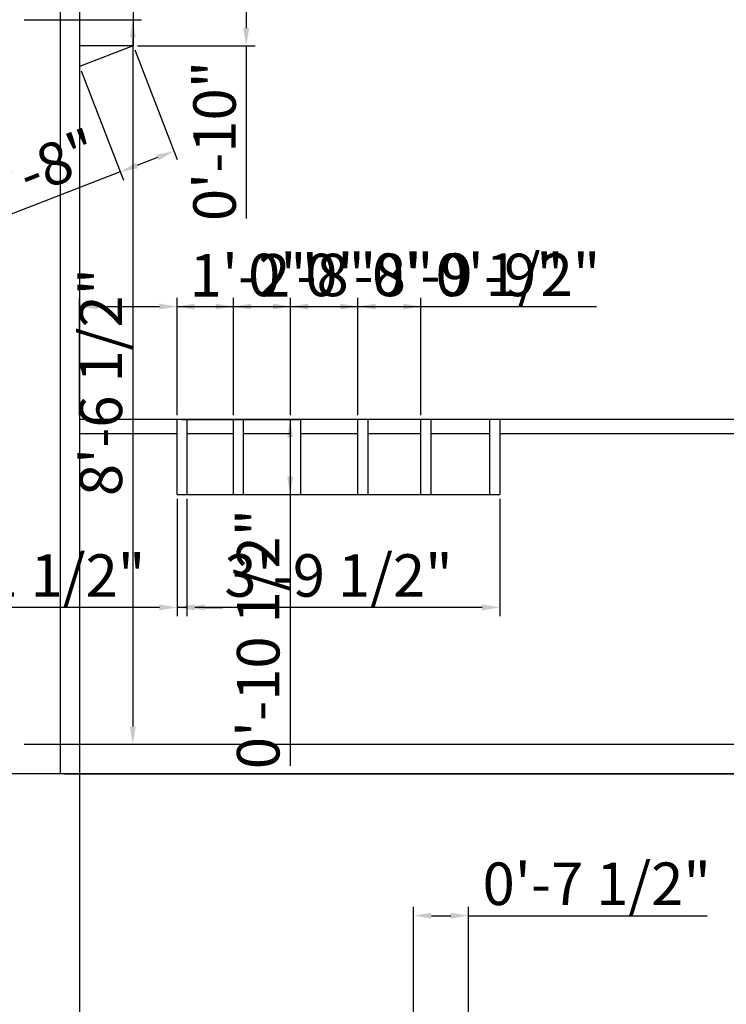
# Model space of a CAD drawing. Units: inches. Extents: x 2656 to 9931, y 1941 to 3068.
# Tile 42 of 46: x 2868 to 2968, y 2855 to 2994. Entities that reach past the tile are written whole.
import ezdxf

# ---------------------------------------------------------------- set-up
doc = ezdxf.new("R2010")
doc.units = ezdxf.units.IN
doc.layers.add('A-ANNO-DIMS', color=2, linetype='Continuous', lineweight=18)
doc.layers.add('A-ELEV', color=7, linetype='Continuous', lineweight=25)
doc.styles.get("Standard").update_dxf_attribs({"font": 'arial.ttf'})
doc.dimstyles.new('ISO-25', dxfattribs={"dimtxt": 6, "dimasz": 2.5, "dimexe": 1.25, "dimexo": 0.625, "dimtad": 1, "dimdec": 0, "dimlunit": 3, "dimtxsty": 'Standard', "dimcen": 2.5, "dimadec": 0, "dimazin": 0, "dimtfac": 1, "dimtdec": 0, "dimtmove": 0, "dimatfit": 3, "dimfxl": 1, "dimarcsym": 0})

# ---------------------------------------------------------------- blocks, each defined once
blk = doc.blocks.new('*D85')
at = {"layer": 'A-ANNO-DIMS', "color": 0, "lineweight": -2, "transparency": 16777216}
for p, q in [((2876.66, 3001.14), (2876.66, 3017.72)), ((3014.98, 2938.52), (3014.98, 3017.72)), ((2879.16, 3016.47), (3012.48, 3016.47))]:
    blk.add_line(p, q, dxfattribs=at)
at = {"layer": 'A-ANNO-DIMS', "color": 0, "transparency": 16777216}
for points in [[(2879.16, 3016.88), (2879.16, 3016.05), (2876.66, 3016.47)], [(3012.48, 3016.88), (3012.48, 3016.05), (3014.98, 3016.47)]]:
    blk.add_solid(points, dxfattribs=at)
at = {"layer": 'Defpoints', "color": 0, "transparency": 16777216}
for p in [(3014.98, 3016.47), (2876.66, 3000.52), (3014.98, 2937.89)]:
    blk.add_point(p, dxfattribs=at)
at = {"layer": 'A-ANNO-DIMS', "color": 0, "transparency": 16777216, "insert": (2945.82, 3020.19), "char_height": 6, "attachment_point": 5}
blk.add_mtext('11\'-6 1/2"', dxfattribs=at)
blk = doc.blocks.new('*D86')
at = {"layer": 'A-ANNO-DIMS', "color": 0, "lineweight": -2, "transparency": 16777216}
for p, q in [((2923.8, 2852.52), (2923.8, 2869.09)), ((2931.54, 2852.52), (2931.54, 2869.09)), ((2926.3, 2867.84), (2929.04, 2867.84)), ((2931.54, 2867.84), (2965.22, 2867.84))]:
    blk.add_line(p, q, dxfattribs=at)
at = {"layer": 'A-ANNO-DIMS', "color": 0, "transparency": 16777216}
for points in [[(2926.3, 2868.26), (2926.3, 2867.43), (2923.8, 2867.84)], [(2929.04, 2868.26), (2929.04, 2867.43), (2931.54, 2867.84)]]:
    blk.add_solid(points, dxfattribs=at)
at = {"layer": 'Defpoints', "color": 0, "transparency": 16777216}
for p in [(2931.54, 2867.84), (2923.8, 2851.89), (2931.54, 2851.89)]:
    blk.add_point(p, dxfattribs=at)
at = {"layer": 'A-ANNO-DIMS', "color": 0, "transparency": 16777216, "insert": (2949.63, 2871.57), "char_height": 6, "attachment_point": 5}
blk.add_mtext('0\'-7 1/2"', dxfattribs=at)
blk = doc.blocks.new('*D149')
at = {"layer": 'A-ANNO-DIMS', "color": 0, "lineweight": -2, "transparency": 16777216}
for p, q in [((2868.85, 2994.35), (2885.43, 2994.35)), ((2884.18, 2991.85), (2884.18, 2894.54)), ((2868.85, 2892.04), (2885.43, 2892.04))]:
    blk.add_line(p, q, dxfattribs=at)
at = {"layer": 'A-ANNO-DIMS', "color": 0, "transparency": 16777216}
for points in [[(2883.76, 2991.85), (2884.59, 2991.85), (2884.18, 2994.35)], [(2883.76, 2894.54), (2884.59, 2894.54), (2884.18, 2892.04)]]:
    blk.add_solid(points, dxfattribs=at)
at = {"layer": 'Defpoints', "color": 0, "transparency": 16777216}
for p in [(2868.23, 2994.35), (2868.23, 2892.04), (2884.18, 2892.04)]:
    blk.add_point(p, dxfattribs=at)
at = {"layer": 'A-ANNO-DIMS', "color": 0, "transparency": 16777216, "insert": (2880.45, 2943.19), "char_height": 6, "attachment_point": 5, "rotation": 90}
blk.add_mtext('8\'-6 1/2"', dxfattribs=at)
blk = doc.blocks.new('*D150')
at = {"layer": 'A-ANNO-DIMS', "color": 0, "lineweight": -2, "transparency": 16777216}
for p, q in [((3046.11, 2894.54), (3046.11, 2897.04)), ((2868.85, 2892.04), (3047.36, 2892.04)), ((3046.11, 2892.04), (3046.11, 2887.89)), ((2874.53, 2887.89), (3047.36, 2887.89)), ((3046.11, 2885.39), (3046.11, 2865.69))]:
    blk.add_line(p, q, dxfattribs=at)
at = {"layer": 'A-ANNO-DIMS', "color": 0, "transparency": 16777216}
for points in [[(3045.69, 2894.54), (3046.53, 2894.54), (3046.11, 2892.04)], [(3045.69, 2885.39), (3046.53, 2885.39), (3046.11, 2887.89)]]:
    blk.add_solid(points, dxfattribs=at)
at = {"layer": 'Defpoints', "color": 0, "transparency": 16777216}
for p in [(2868.23, 2892.04), (2873.91, 2887.89), (3046.11, 2887.89)]:
    blk.add_point(p, dxfattribs=at)
at = {"layer": 'A-ANNO-DIMS', "color": 0, "transparency": 16777216, "insert": (3042.42, 2874.29), "char_height": 6, "attachment_point": 5, "rotation": 90}
blk.add_mtext('0\'-4"', dxfattribs=at)
blk = doc.blocks.new('*D156')
at = {"layer": 'A-ANNO-DIMS', "color": 0, "lineweight": -2, "transparency": 16777216}
for p, q in [((2876.66, 2938.52), (2876.66, 2955.09)), ((2890.43, 2938.52), (2890.43, 2955.09)), ((2879.16, 2953.84), (2887.93, 2953.84)), ((2890.43, 2953.84), (2909.56, 2953.84))]:
    blk.add_line(p, q, dxfattribs=at)
at = {"layer": 'A-ANNO-DIMS', "color": 0, "transparency": 16777216}
for points in [[(2879.16, 2954.26), (2879.16, 2953.43), (2876.66, 2953.84)], [(2887.93, 2954.26), (2887.93, 2953.43), (2890.43, 2953.84)]]:
    blk.add_solid(points, dxfattribs=at)
at = {"layer": 'Defpoints', "color": 0, "transparency": 16777216}
for p in [(2890.43, 2953.84), (2876.66, 2937.89), (2890.43, 2937.89)]:
    blk.add_point(p, dxfattribs=at)
at = {"layer": 'A-ANNO-DIMS', "color": 0, "transparency": 16777216, "insert": (2901.25, 2957.48), "char_height": 6, "attachment_point": 5}
blk.add_mtext('1\'-2"', dxfattribs=at)
blk = doc.blocks.new('*D157')
at = {"layer": 'A-ANNO-DIMS', "color": 0, "lineweight": -2, "transparency": 16777216}
for p, q in [((2890.43, 2926.69), (2890.43, 2910.12)), ((2935.96, 2926.69), (2935.96, 2910.12)), ((2933.46, 2911.37), (2892.93, 2911.37))]:
    blk.add_line(p, q, dxfattribs=at)
at = {"layer": 'A-ANNO-DIMS', "color": 0, "transparency": 16777216}
for points in [[(2892.93, 2911.78), (2892.93, 2910.95), (2890.43, 2911.37)], [(2933.46, 2911.78), (2933.46, 2910.95), (2935.96, 2911.37)]]:
    blk.add_solid(points, dxfattribs=at)
at = {"layer": 'Defpoints', "color": 0, "transparency": 16777216}
for p in [(2890.43, 2927.32), (2935.96, 2927.32), (2890.43, 2911.37)]:
    blk.add_point(p, dxfattribs=at)
at = {"layer": 'A-ANNO-DIMS', "color": 0, "transparency": 16777216, "insert": (2913.2, 2915.1), "char_height": 6, "attachment_point": 5}
blk.add_mtext('3\'-9 1/2"', dxfattribs=at)
blk = doc.blocks.new('*D158')
at = {"layer": 'A-ANNO-DIMS', "color": 0, "lineweight": -2, "transparency": 16777216}
for p, q in [((2891.05, 2937.89), (2907.63, 2937.89)), ((2906.38, 2935.39), (2906.38, 2929.82)), ((2891.05, 2927.32), (2907.63, 2927.32)), ((2906.38, 2927.32), (2906.38, 2888.98))]:
    blk.add_line(p, q, dxfattribs=at)
at = {"layer": 'A-ANNO-DIMS', "color": 0, "transparency": 16777216}
for points in [[(2905.96, 2935.39), (2906.79, 2935.39), (2906.38, 2937.89)], [(2905.96, 2929.82), (2906.79, 2929.82), (2906.38, 2927.32)]]:
    blk.add_solid(points, dxfattribs=at)
at = {"layer": 'Defpoints', "color": 0, "transparency": 16777216}
for p in [(2890.43, 2937.89), (2890.43, 2927.32), (2906.38, 2927.32)]:
    blk.add_point(p, dxfattribs=at)
at = {"layer": 'A-ANNO-DIMS', "color": 0, "transparency": 16777216, "insert": (2902.65, 2906.9), "char_height": 6, "attachment_point": 5, "rotation": 90}
blk.add_mtext('0\'-10 1/2"', dxfattribs=at)
blk = doc.blocks.new('*D159')
at = {"layer": 'A-ANNO-DIMS', "color": 0, "lineweight": -2, "transparency": 16777216}
for p, q in [((2890.43, 2938.52), (2890.43, 2955.09)), ((2898.38, 2938.52), (2898.38, 2955.09)), ((2892.93, 2953.84), (2895.88, 2953.84)), ((2898.38, 2953.84), (2918.08, 2953.84))]:
    blk.add_line(p, q, dxfattribs=at)
at = {"layer": 'A-ANNO-DIMS', "color": 0, "transparency": 16777216}
for points in [[(2892.93, 2954.26), (2892.93, 2953.43), (2890.43, 2953.84)], [(2895.88, 2954.26), (2895.88, 2953.43), (2898.38, 2953.84)]]:
    blk.add_solid(points, dxfattribs=at)
at = {"layer": 'Defpoints', "color": 0, "transparency": 16777216}
for p in [(2898.38, 2953.84), (2890.43, 2937.89), (2898.38, 2937.89)]:
    blk.add_point(p, dxfattribs=at)
at = {"layer": 'A-ANNO-DIMS', "color": 0, "transparency": 16777216, "insert": (2909.48, 2957.53), "char_height": 6, "attachment_point": 5}
blk.add_mtext('0\'-8"', dxfattribs=at)
blk = doc.blocks.new('*D160')
at = {"layer": 'A-ANNO-DIMS', "color": 0, "lineweight": -2, "transparency": 16777216}
for p, q in [((2898.38, 2938.52), (2898.38, 2955.09)), ((2906.45, 2938.52), (2906.45, 2955.09)), ((2900.88, 2953.84), (2903.95, 2953.84)), ((2906.45, 2953.84), (2926.15, 2953.84))]:
    blk.add_line(p, q, dxfattribs=at)
at = {"layer": 'A-ANNO-DIMS', "color": 0, "transparency": 16777216}
for points in [[(2900.88, 2954.26), (2900.88, 2953.43), (2898.38, 2953.84)], [(2903.95, 2954.26), (2903.95, 2953.43), (2906.45, 2953.84)]]:
    blk.add_solid(points, dxfattribs=at)
at = {"layer": 'Defpoints', "color": 0, "transparency": 16777216}
for p in [(2906.45, 2953.84), (2898.38, 2937.89), (2906.45, 2937.89)]:
    blk.add_point(p, dxfattribs=at)
at = {"layer": 'A-ANNO-DIMS', "color": 0, "transparency": 16777216, "insert": (2917.55, 2957.53), "char_height": 6, "attachment_point": 5}
blk.add_mtext('0\'-8"', dxfattribs=at)
blk = doc.blocks.new('*D161')
at = {"layer": 'A-ANNO-DIMS', "color": 0, "lineweight": -2, "transparency": 16777216}
for p, q in [((2906.45, 2938.52), (2906.45, 2955.09)), ((2915.94, 2938.52), (2915.94, 2955.09)), ((2908.95, 2953.84), (2913.44, 2953.84)), ((2915.94, 2953.84), (2949.62, 2953.84))]:
    blk.add_line(p, q, dxfattribs=at)
at = {"layer": 'A-ANNO-DIMS', "color": 0, "transparency": 16777216}
for points in [[(2908.95, 2954.26), (2908.95, 2953.43), (2906.45, 2953.84)], [(2913.44, 2954.26), (2913.44, 2953.43), (2915.94, 2953.84)]]:
    blk.add_solid(points, dxfattribs=at)
at = {"layer": 'Defpoints', "color": 0, "transparency": 16777216}
for p in [(2915.94, 2953.84), (2906.45, 2937.89), (2915.94, 2937.89)]:
    blk.add_point(p, dxfattribs=at)
at = {"layer": 'A-ANNO-DIMS', "color": 0, "transparency": 16777216, "insert": (2934.03, 2957.57), "char_height": 6, "attachment_point": 5}
blk.add_mtext('0\'-9 1/2"', dxfattribs=at)
blk = doc.blocks.new('*D162')
at = {"layer": 'A-ANNO-DIMS', "color": 0, "lineweight": -2, "transparency": 16777216}
for p, q in [((2915.94, 2938.52), (2915.94, 2955.09)), ((2924.83, 2938.52), (2924.83, 2955.09)), ((2918.44, 2953.84), (2922.33, 2953.84)), ((2924.83, 2953.84), (2944.53, 2953.84))]:
    blk.add_line(p, q, dxfattribs=at)
at = {"layer": 'A-ANNO-DIMS', "color": 0, "transparency": 16777216}
for points in [[(2918.44, 2954.26), (2918.44, 2953.43), (2915.94, 2953.84)], [(2922.33, 2954.26), (2922.33, 2953.43), (2924.83, 2953.84)]]:
    blk.add_solid(points, dxfattribs=at)
at = {"layer": 'Defpoints', "color": 0, "transparency": 16777216}
for p in [(2924.83, 2953.84), (2915.94, 2937.89), (2924.83, 2937.89)]:
    blk.add_point(p, dxfattribs=at)
at = {"layer": 'A-ANNO-DIMS', "color": 0, "transparency": 16777216, "insert": (2935.93, 2957.53), "char_height": 6, "attachment_point": 5}
blk.add_mtext('0\'-9"', dxfattribs=at)
blk = doc.blocks.new('*D163')
at = {"layer": 'A-ANNO-DIMS', "color": 0, "lineweight": -2, "transparency": 16777216}
for p, q in [((2890.43, 2926.69), (2890.43, 2910.12)), ((2891.82, 2926.69), (2891.82, 2910.12)), ((2887.93, 2911.37), (2854.25, 2911.37)), ((2891.82, 2911.37), (2890.43, 2911.37)), ((2894.32, 2911.37), (2896.82, 2911.37))]:
    blk.add_line(p, q, dxfattribs=at)
at = {"layer": 'A-ANNO-DIMS', "color": 0, "transparency": 16777216}
for points in [[(2887.93, 2911.78), (2887.93, 2910.95), (2890.43, 2911.37)], [(2894.32, 2911.78), (2894.32, 2910.95), (2891.82, 2911.37)]]:
    blk.add_solid(points, dxfattribs=at)
at = {"layer": 'Defpoints', "color": 0, "transparency": 16777216}
for p in [(2890.43, 2927.32), (2891.82, 2927.32), (2890.43, 2911.37)]:
    blk.add_point(p, dxfattribs=at)
at = {"layer": 'A-ANNO-DIMS', "color": 0, "transparency": 16777216, "insert": (2869.84, 2915.09), "char_height": 6, "attachment_point": 5}
blk.add_mtext('0\'-1 1/2"', dxfattribs=at)
blk = doc.blocks.new('*D165')
at = {"layer": 'A-ANNO-DIMS', "color": 0, "lineweight": -2, "transparency": 16777216}
for p, q in [((2884.85, 3000.52), (2901.43, 3000.52)), ((2900.18, 2998.02), (2900.18, 2993.16)), ((2884.85, 2990.66), (2901.43, 2990.66)), ((2900.18, 2990.66), (2900.18, 2966.3))]:
    blk.add_line(p, q, dxfattribs=at)
at = {"layer": 'A-ANNO-DIMS', "color": 0, "transparency": 16777216}
for points in [[(2899.76, 2998.02), (2900.6, 2998.02), (2900.18, 3000.52)], [(2899.76, 2993.16), (2900.6, 2993.16), (2900.18, 2990.66)]]:
    blk.add_solid(points, dxfattribs=at)
at = {"layer": 'Defpoints', "color": 0, "transparency": 16777216}
for p in [(2884.23, 3000.52), (2884.23, 2990.66), (2900.18, 2990.66)]:
    blk.add_point(p, dxfattribs=at)
at = {"layer": 'A-ANNO-DIMS', "color": 0, "transparency": 16777216, "insert": (2896.49, 2977.23), "char_height": 6, "attachment_point": 5, "rotation": 90}
blk.add_mtext('0\'-10"', dxfattribs=at)
blk = doc.blocks.new('*D166')
at = {"layer": 'A-ANNO-DIMS', "color": 0, "lineweight": -2, "transparency": 16777216}
for p, q in [((2884.45, 2990.07), (2890.44, 2974.62)), ((2876.88, 2987.15), (2882.86, 2971.69)), ((2887.65, 2974.88), (2884.74, 2973.75)), ((2882.41, 2972.85), (2864.04, 2965.74))]:
    blk.add_line(p, q, dxfattribs=at)
at = {"layer": 'A-ANNO-DIMS', "color": 0, "transparency": 16777216}
for points in [[(2887.5, 2975.27), (2887.8, 2974.49), (2889.98, 2975.78)], [(2884.59, 2974.14), (2884.89, 2973.37), (2882.41, 2972.85)]]:
    blk.add_solid(points, dxfattribs=at)
at = {"layer": 'Defpoints', "color": 0, "transparency": 16777216}
for p in [(2884.23, 2990.66), (2876.66, 2987.73), (2882.41, 2972.85)]:
    blk.add_point(p, dxfattribs=at)
at = {"layer": 'A-ANNO-DIMS', "color": 0, "transparency": 16777216, "insert": (2870.73, 2972.29), "char_height": 6, "attachment_point": 5, "rotation": 21.1508}
blk.add_mtext('0\'-8"', dxfattribs=at)

msp = doc.modelspace()

# ---------------------------------------------------------------- linework, layer by layer
at = {"layer": 'A-ELEV'}
for p, q in [((2876.66, 3000.52), (2876.66, 2935.89)), ((2884.23, 3000.52), (2884.23, 2990.66)), ((2884.23, 2990.66), (2876.66, 2990.66)), ((2884.23, 2990.66), (2876.66, 2987.73)), ((2998.16, 2937.89), (2876.66, 2937.89)), ((2890.43, 2927.32), (2890.43, 2937.89)), ((2891.82, 2937.89), (2891.82, 2927.32)), ((2898.38, 2927.32), (2898.38, 2937.89)), ((2899.77, 2937.89), (2899.77, 2927.32)), ((2906.45, 2927.32), (2906.45, 2937.89)), ((2907.84, 2937.89), (2907.84, 2927.32)), ((2915.94, 2927.32), (2915.94, 2937.89)), ((2917.33, 2937.89), (2917.33, 2927.32)), ((2924.83, 2927.32), (2924.83, 2937.89)), ((2926.22, 2937.89), (2926.22, 2927.32)), ((2934.57, 2927.32), (2934.57, 2937.89)), ((2935.96, 2937.89), (2935.96, 2927.32)), ((2876.66, 2935.89), (2876.66, 2893.89)), ((2890.43, 2935.89), (2876.66, 2935.89)), ((2898.38, 2935.89), (2891.82, 2935.89)), ((2906.45, 2935.89), (2899.77, 2935.89)), ((2915.94, 2935.89), (2907.84, 2935.89)), ((2924.83, 2935.89), (2917.33, 2935.89)), ((2934.57, 2935.89), (2926.22, 2935.89)), ((2998.16, 2935.89), (2935.96, 2935.89)), ((2890.43, 2927.32), (2935.96, 2927.32)), ((2873.91, 2898.94), (2873.91, 2887.89)), ((2876.66, 2893.89), (2876.66, 2887.89)), ((2998.16, 2887.89), (2743.16, 2887.89)), ((2876.66, 2887.89), (2876.66, 2797.89))]:
    msp.add_line(p, q, dxfattribs=at)
msp.add_lwpolyline([(2873.91, 3000.52), (2873.91, 2898.94)], dxfattribs=at)

# ---------------------------------------------------------------- dimensions: what is measured, and where the dimension line sits
at = {"layer": 'A-ANNO-DIMS'}
for base, p1, p2, picture, middle in [((3014.98, 3016.47), (2876.66, 3000.52), (3014.98, 2937.89), '*D85', (2945.82, 3020.19)), ((2915.94, 2953.84), (2906.45, 2937.89), (2915.94, 2937.89), '*D161', (2934.03, 2957.57)), ((2890.43, 2953.84), (2876.66, 2937.89), (2890.43, 2937.89), '*D156', (2901.25, 2957.48)), ((2898.3756, 2953.8431), (2890.428, 2937.8931), (2898.3756, 2937.8931), '*D159', (2909.4754, 2957.5315)), ((2906.45, 2953.84), (2898.38, 2937.89), (2906.45, 2937.89), '*D160', (2917.55, 2957.53)), ((2924.83, 2953.84), (2915.94, 2937.89), (2924.83, 2937.89), '*D162', (2935.93, 2957.53)), ((2931.54, 2867.84), (2923.8, 2851.89), (2931.54, 2851.89), '*D86', (2949.63, 2871.57))]:
    dim = msp.add_linear_dim(base=base, p1=p1, p2=p2, dimstyle='ISO-25', override={"dimdec": 1, "dimlfac": 1, "dimrnd": 0, "dimzin": 1, "dimdsep": 46, "dimlunit": 4, "dimfrac": 2}, dxfattribs=at)
    dim.commit()
    dim.dimension.update_dxf_attribs({"geometry": picture, "text_midpoint": middle})
for base, p1, p2, angle, picture, middle in [((2900.18, 2990.66), (2884.23, 3000.52), (2884.23, 2990.66), 270, '*D165', (2896.49, 2977.23)), ((2884.18, 2892.04), (2868.23, 2994.35), (2868.23, 2892.04), 270, '*D149', (2880.45, 2943.19)), ((2882.41, 2972.85), (2884.23, 2990.66), (2876.66, 2987.73), 201.1508, '*D166', (2870.73, 2972.29)), ((2906.38, 2927.32), (2890.43, 2937.89), (2890.43, 2927.32), 270, '*D158', (2902.65, 2906.9)), ((2890.43, 2911.37), (2891.82, 2927.32), (2890.43, 2927.32), 180, '*D163', (2869.84, 2915.09)), ((2890.43, 2911.37), (2935.96, 2927.32), (2890.43, 2927.32), 180, '*D157', (2913.2, 2915.1)), ((3046.11, 2887.8931), (2868.2256, 2892.0351), (2873.907, 2887.8931), 90, '*D150', (3042.4215, 2874.2933))]:
    dim = msp.add_linear_dim(base=base, p1=p1, p2=p2, angle=angle, dimstyle='ISO-25', override={"dimdec": 1, "dimlfac": 1, "dimrnd": 0, "dimzin": 1, "dimdsep": 46, "dimlunit": 4, "dimfrac": 2}, dxfattribs=at)
    dim.commit()
    dim.dimension.update_dxf_attribs({"geometry": picture, "text_midpoint": middle})

doc.saveas('drawing.dxf')
